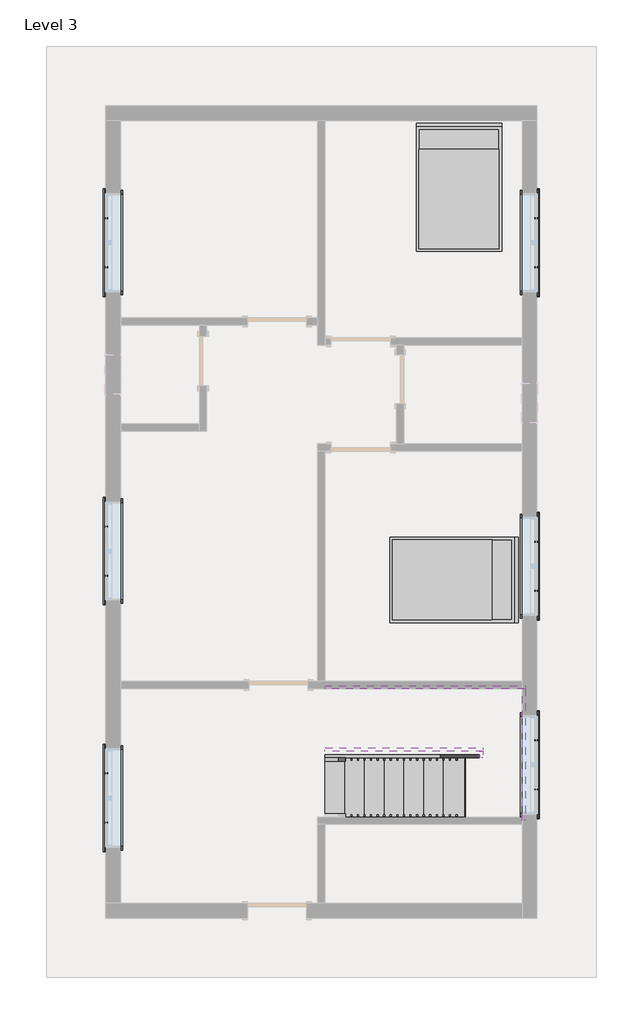
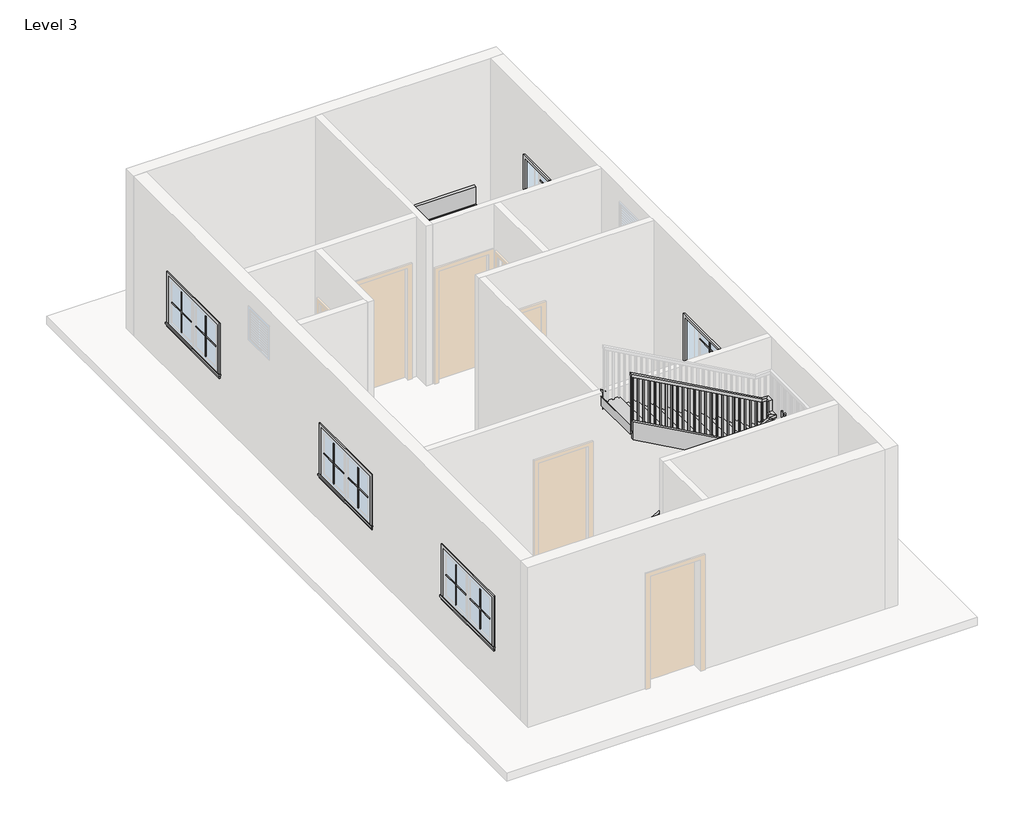
# One storey, part 3 of 3: 24 proxies, 6 members, 2 furniture elements, 1 railing, 1 stair flight.
"""IFC4 building model written with IfcOpenShell, lengths in millimetres."""

from ifc_helpers import new_model, si_unit, frame, origin, place, context, project, spatial, polyline, outline, extrude, faceted_brep, transform, mapped, element, save
from components import muntin_pattern_2x2_muntin_pattern_2x2_9352d081, muntin_pattern_2x2_muntin_pattern_2x2_5c2cbe28, trim_window_exterior_flat_with_sill_979bde60, trim_window_interior_flat_picture_frame_7883d11b, bed_17739_bed_17739_15c61121, stair_flight_460b4896

model = new_model("IFC4")

# Units and contexts
model_context = context("Model", 3, world=origin())
ifc_project = project(units=[si_unit("LENGTHUNIT", "METRE", prefix="MILLI")], contexts=[model_context])

# Site, building, storey
site = spatial("IfcSite", under=ifc_project)
building = spatial("IfcBuilding", under=site)
storey = spatial("IfcBuildingStorey", under=building, Name="Level 3", Elevation=6248.4)

# Proxies
placement = place(None, origin())
muntin_pattern_2x2_muntin_pattern_2x2_shape = muntin_pattern_2x2_muntin_pattern_2x2_9352d081(model_context)
element("IfcBuildingElementProxy", 1, Name="Muntin Pattern_2x2 : Muntin Pattern_2x2", ObjectType="Muntin Pattern_2x2 : Muntin Pattern_2x2", at=placement, inside=storey, context=model_context, shape_type="MappedRepresentation", body=[
    mapped(muntin_pattern_2x2_muntin_pattern_2x2_shape, transform((-4579.34688, 3675.02881, 7232.65), x_axis=(0.0, 1.0, 0.0), y_axis=(-1.0, 0.0, 0.0), z_axis=(0.0, 0.0, 1.0))),
])
element("IfcBuildingElementProxy", 2, Name="Muntin Pattern_2x2 : Muntin Pattern_2x2", ObjectType="Muntin Pattern_2x2 : Muntin Pattern_2x2", at=placement, inside=storey, context=model_context, shape_type="MappedRepresentation", body=[
    mapped(muntin_pattern_2x2_muntin_pattern_2x2_shape, transform((-4579.34688, -1087.47119, 7232.65), x_axis=(0.0, 1.0, 0.0), y_axis=(-1.0, 0.0, 0.0), z_axis=(0.0, 0.0, 1.0))),
])
element("IfcBuildingElementProxy", 3, Name="Muntin Pattern_2x2 : Muntin Pattern_2x2", ObjectType="Muntin Pattern_2x2 : Muntin Pattern_2x2", at=placement, inside=storey, context=model_context, shape_type="MappedRepresentation", body=[
    mapped(muntin_pattern_2x2_muntin_pattern_2x2_shape, transform((-4579.34688, -4900.64619, 7232.65), x_axis=(0.0, 1.0, 0.0), y_axis=(-1.0, 0.0, 0.0), z_axis=(0.0, 0.0, 1.0))),
])
element("IfcBuildingElementProxy", 4, Name="Muntin Pattern_2x2 : Muntin Pattern_2x2", ObjectType="Muntin Pattern_2x2 : Muntin Pattern_2x2", at=placement, inside=storey, context=model_context, shape_type="MappedRepresentation", body=[
    mapped(muntin_pattern_2x2_muntin_pattern_2x2_shape, transform((2069.10312, -3630.64619, 7232.65), x_axis=(0.0, -1.0, 0.0), y_axis=(1.0, 0.0, 0.0), z_axis=(0.0, 0.0, 1.0))),
])
element("IfcBuildingElementProxy", 5, Name="Muntin Pattern_2x2 : Muntin Pattern_2x2", ObjectType="Muntin Pattern_2x2 : Muntin Pattern_2x2", at=placement, inside=storey, context=model_context, shape_type="MappedRepresentation", body=[
    mapped(muntin_pattern_2x2_muntin_pattern_2x2_shape, transform((2069.10312, 4433.85381, 7232.65), x_axis=(0.0, -1.0, 0.0), y_axis=(1.0, 0.0, 0.0), z_axis=(0.0, 0.0, 1.0))),
])
element("IfcBuildingElementProxy", 6, Name="Muntin Pattern_2x2 : Muntin Pattern_2x2", ObjectType="Muntin Pattern_2x2 : Muntin Pattern_2x2", at=placement, inside=storey, context=model_context, shape_type="MappedRepresentation", body=[
    mapped(muntin_pattern_2x2_muntin_pattern_2x2_shape, transform((2069.10312, -563.59619, 7232.65), x_axis=(0.0, -1.0, 0.0), y_axis=(1.0, 0.0, 0.0), z_axis=(0.0, 0.0, 1.0))),
])
muntin_pattern_2x2_muntin_pattern_2x2_2_shape = muntin_pattern_2x2_muntin_pattern_2x2_5c2cbe28(model_context)
element("IfcBuildingElementProxy", 7, Name="Muntin Pattern_2x2 : Muntin Pattern_2x2", ObjectType="Muntin Pattern_2x2 : Muntin Pattern_2x2", at=placement, inside=storey, context=model_context, shape_type="MappedRepresentation", body=[
    mapped(muntin_pattern_2x2_muntin_pattern_2x2_2_shape, transform((-4579.34688, 4433.85381, 7232.65), x_axis=(0.0, -1.0, 0.0), y_axis=(1.0, 0.0, 0.0), z_axis=(0.0, 0.0, 1.0))),
])
element("IfcBuildingElementProxy", 8, Name="Muntin Pattern_2x2 : Muntin Pattern_2x2", ObjectType="Muntin Pattern_2x2 : Muntin Pattern_2x2", at=placement, inside=storey, context=model_context, shape_type="MappedRepresentation", body=[
    mapped(muntin_pattern_2x2_muntin_pattern_2x2_2_shape, transform((-4579.34688, -328.64619, 7232.65), x_axis=(0.0, -1.0, 0.0), y_axis=(1.0, 0.0, 0.0), z_axis=(0.0, 0.0, 1.0))),
])
element("IfcBuildingElementProxy", 9, Name="Muntin Pattern_2x2 : Muntin Pattern_2x2", ObjectType="Muntin Pattern_2x2 : Muntin Pattern_2x2", at=placement, inside=storey, context=model_context, shape_type="MappedRepresentation", body=[
    mapped(muntin_pattern_2x2_muntin_pattern_2x2_2_shape, transform((-4579.34688, -4141.82119, 7232.65), x_axis=(0.0, -1.0, 0.0), y_axis=(1.0, 0.0, 0.0), z_axis=(0.0, 0.0, 1.0))),
])
element("IfcBuildingElementProxy", 10, Name="Muntin Pattern_2x2 : Muntin Pattern_2x2", ObjectType="Muntin Pattern_2x2 : Muntin Pattern_2x2", at=placement, inside=storey, context=model_context, shape_type="MappedRepresentation", body=[
    mapped(muntin_pattern_2x2_muntin_pattern_2x2_2_shape, transform((2069.10312, -4389.47119, 7232.65), x_axis=(0.0, 1.0, 0.0), y_axis=(-1.0, 0.0, 0.0), z_axis=(0.0, 0.0, 1.0))),
])
element("IfcBuildingElementProxy", 11, Name="Muntin Pattern_2x2 : Muntin Pattern_2x2", ObjectType="Muntin Pattern_2x2 : Muntin Pattern_2x2", at=placement, inside=storey, context=model_context, shape_type="MappedRepresentation", body=[
    mapped(muntin_pattern_2x2_muntin_pattern_2x2_2_shape, transform((2069.10312, 3675.02881, 7232.65), x_axis=(0.0, 1.0, 0.0), y_axis=(-1.0, 0.0, 0.0), z_axis=(0.0, 0.0, 1.0))),
])
element("IfcBuildingElementProxy", 12, Name="Muntin Pattern_2x2 : Muntin Pattern_2x2", ObjectType="Muntin Pattern_2x2 : Muntin Pattern_2x2", at=placement, inside=storey, context=model_context, shape_type="MappedRepresentation", body=[
    mapped(muntin_pattern_2x2_muntin_pattern_2x2_2_shape, transform((2069.10312, -1322.42119, 7232.65), x_axis=(0.0, 1.0, 0.0), y_axis=(-1.0, 0.0, 0.0), z_axis=(0.0, 0.0, 1.0))),
])
trim_window_exterior_flat_with_sill_shape = trim_window_exterior_flat_with_sill_979bde60(model_context)
element("IfcBuildingElementProxy", 13, Name="Trim-Window-Exterior-Flat : with Sill", ObjectType="Trim-Window-Exterior-Flat : with Sill", at=placement, inside=storey, context=model_context, shape_type="MappedRepresentation", body=[
    mapped(trim_window_exterior_flat_with_sill_shape, transform((-4588.87188, 4054.44131, 8077.2), x_axis=(0.0, -1.0, 0.0), y_axis=(0.0, 0.0, 1.0), z_axis=(-1.0, 0.0, 0.0))),
])
element("IfcBuildingElementProxy", 14, Name="Trim-Window-Exterior-Flat : with Sill", ObjectType="Trim-Window-Exterior-Flat : with Sill", at=placement, inside=storey, context=model_context, shape_type="MappedRepresentation", body=[
    mapped(trim_window_exterior_flat_with_sill_shape, transform((-4588.87188, -708.05869, 8077.2), x_axis=(0.0, -1.0, 0.0), y_axis=(0.0, 0.0, 1.0), z_axis=(-1.0, 0.0, 0.0))),
])
element("IfcBuildingElementProxy", 15, Name="Trim-Window-Exterior-Flat : with Sill", ObjectType="Trim-Window-Exterior-Flat : with Sill", at=placement, inside=storey, context=model_context, shape_type="MappedRepresentation", body=[
    mapped(trim_window_exterior_flat_with_sill_shape, transform((-4588.87188, -4521.23369, 8077.2), x_axis=(0.0, -1.0, 0.0), y_axis=(0.0, 0.0, 1.0), z_axis=(-1.0, 0.0, 0.0))),
])
element("IfcBuildingElementProxy", 16, Name="Trim-Window-Exterior-Flat : with Sill", ObjectType="Trim-Window-Exterior-Flat : with Sill", at=placement, inside=storey, context=model_context, shape_type="MappedRepresentation", body=[
    mapped(trim_window_exterior_flat_with_sill_shape, transform((2078.62812, -4010.05869, 8077.2), x_axis=(0.0, 1.0, 0.0), y_axis=(0.0, 0.0, 1.0), z_axis=(1.0, 0.0, 0.0))),
])
element("IfcBuildingElementProxy", 17, Name="Trim-Window-Exterior-Flat : with Sill", ObjectType="Trim-Window-Exterior-Flat : with Sill", at=placement, inside=storey, context=model_context, shape_type="MappedRepresentation", body=[
    mapped(trim_window_exterior_flat_with_sill_shape, transform((2078.62812, 4054.44131, 8077.2), x_axis=(0.0, 1.0, 0.0), y_axis=(0.0, 0.0, 1.0), z_axis=(1.0, 0.0, 0.0))),
])
element("IfcBuildingElementProxy", 18, Name="Trim-Window-Exterior-Flat : with Sill", ObjectType="Trim-Window-Exterior-Flat : with Sill", at=placement, inside=storey, context=model_context, shape_type="MappedRepresentation", body=[
    mapped(trim_window_exterior_flat_with_sill_shape, transform((2078.62812, -943.00869, 8077.2), x_axis=(0.0, 1.0, 0.0), y_axis=(0.0, 0.0, 1.0), z_axis=(1.0, 0.0, 0.0))),
])
trim_window_interior_flat_picture_frame_shape = trim_window_interior_flat_picture_frame_7883d11b(model_context)
element("IfcBuildingElementProxy", 19, Name="Trim-Window-Interior-Flat : Picture Frame", ObjectType="Trim-Window-Interior-Flat : Picture Frame", at=placement, inside=storey, context=model_context, shape_type="MappedRepresentation", body=[
    mapped(trim_window_interior_flat_picture_frame_shape, transform((-4360.27188, 4054.44131, 8077.2), x_axis=(0.0, 1.0, 0.0), y_axis=(0.0, 0.0, 1.0), z_axis=(1.0, 0.0, 0.0))),
])
element("IfcBuildingElementProxy", 20, Name="Trim-Window-Interior-Flat : Picture Frame", ObjectType="Trim-Window-Interior-Flat : Picture Frame", at=placement, inside=storey, context=model_context, shape_type="MappedRepresentation", body=[
    mapped(trim_window_interior_flat_picture_frame_shape, transform((-4360.27188, -708.05869, 8077.2), x_axis=(0.0, 1.0, 0.0), y_axis=(0.0, 0.0, 1.0), z_axis=(1.0, 0.0, 0.0))),
])
element("IfcBuildingElementProxy", 21, Name="Trim-Window-Interior-Flat : Picture Frame", ObjectType="Trim-Window-Interior-Flat : Picture Frame", at=placement, inside=storey, context=model_context, shape_type="MappedRepresentation", body=[
    mapped(trim_window_interior_flat_picture_frame_shape, transform((-4360.27188, -4521.23369, 8077.2), x_axis=(0.0, 1.0, 0.0), y_axis=(0.0, 0.0, 1.0), z_axis=(1.0, 0.0, 0.0))),
])
element("IfcBuildingElementProxy", 22, Name="Trim-Window-Interior-Flat : Picture Frame", ObjectType="Trim-Window-Interior-Flat : Picture Frame", at=placement, inside=storey, context=model_context, shape_type="MappedRepresentation", body=[
    mapped(trim_window_interior_flat_picture_frame_shape, transform((1850.02812, -4010.05869, 8077.2), x_axis=(0.0, -1.0, 0.0), y_axis=(0.0, 0.0, 1.0), z_axis=(-1.0, 0.0, 0.0))),
])
element("IfcBuildingElementProxy", 23, Name="Trim-Window-Interior-Flat : Picture Frame", ObjectType="Trim-Window-Interior-Flat : Picture Frame", at=placement, inside=storey, context=model_context, shape_type="MappedRepresentation", body=[
    mapped(trim_window_interior_flat_picture_frame_shape, transform((1850.02812, 4054.44131, 8077.2), x_axis=(0.0, -1.0, 0.0), y_axis=(0.0, 0.0, 1.0), z_axis=(-1.0, 0.0, 0.0))),
])
element("IfcBuildingElementProxy", 24, Name="Trim-Window-Interior-Flat : Picture Frame", ObjectType="Trim-Window-Interior-Flat : Picture Frame", at=placement, inside=storey, context=model_context, shape_type="MappedRepresentation", body=[
    mapped(trim_window_interior_flat_picture_frame_shape, transform((1850.02812, -943.00869, 8077.2), x_axis=(0.0, -1.0, 0.0), y_axis=(0.0, 0.0, 1.0), z_axis=(-1.0, 0.0, 0.0))),
])

# Furniture
bed_17739_bed_17739_shape = bed_17739_bed_17739_15c61121(model_context)
element("IfcFurniture", 25, ObjectType="Bed_17739 : Bed_17739", at=placement, inside=storey, context=model_context, shape_type="MappedRepresentation", body=[
    mapped(bed_17739_bed_17739_shape, transform((872.12812, 4886.29131, 6248.4), x_axis=(1.0, 0.0, 0.0), y_axis=(0.0, 1.0, 0.0), z_axis=(0.0, 0.0, 1.0))),
])
element("IfcFurniture", 26, ObjectType="Bed_17739 : Bed_17739", at=placement, inside=storey, context=model_context, shape_type="MappedRepresentation", body=[
    mapped(bed_17739_bed_17739_shape, transform((770.52812, -1152.55869, 6248.4), x_axis=(0.0, -1.0, 0.0), y_axis=(1.0, 0.0, 0.0), z_axis=(0.0, 0.0, 1.0))),
])

# Members
element("IfcMember", 27, ObjectType="Stringer - 2\" Width", at=placement, inside=storey, context=model_context, shape_type="SweptSolid", body=[
    extrude(outline(polyline([(6455.9983948, -1197.97188), (6248.4, -1197.97188), (6248.4, -944.0273772), (7433.7641651, 1189.62812), (7782.4428392, 1189.62812), (6455.9983948, -1197.97188)])), frame((0.0, -3902.10869, 0.0), z_axis=(0.0, 1.0, 0.0), x_axis=(0.0, 0.0, 1.0)), (0.0, 0.0, 1.0), 50.8),
])
element("IfcMember", 28, ObjectType="Stringer - 2\" Width", at=placement, inside=storey, context=model_context, shape_type="SweptSolid", body=[
    extrude(outline(polyline([(1240.42812, -3902.10869), (1189.62812, -3902.10869), (1189.62812, -3800.50869), (1240.42812, -3800.50869), (1240.42812, -3902.10869)])), frame((0.0, 0.0, 7543.8), z_axis=(0.0, 0.0, 1.0), x_axis=(1.0, 0.0, 0.0)), (0.0, 0.0, 1.0), 304.8),
])
element("IfcMember", 29, ObjectType="Stringer - 2\" Width", at=placement, inside=storey, context=model_context, shape_type="SweptSolid", body=[
    extrude(outline(polyline([(7631.3197207, 1240.42812), (7979.9983948, 1240.42812), (9334.6650614, -1197.97188), (8985.9863873, -1197.97188), (7631.3197207, 1240.42812)])), frame((0.0, -3800.50869, 0.0), z_axis=(0.0, 1.0, 0.0), x_axis=(0.0, 0.0, 1.0)), (0.0, 0.0, 1.0), 50.8),
])
element("IfcMember", 30, ObjectType="Stringer - 2\" Width", at=placement, inside=storey, context=model_context, shape_type="SweptSolid", body=[
    extrude(outline(polyline([(6455.9983948, -1197.97188), (6248.4, -1197.97188), (6248.4, -944.0273772), (7800.653054, 1850.02812), (7848.6, 1850.02812), (7848.6, 1308.7110094), (6455.9983948, -1197.97188)])), frame((0.0, -4867.30869, 0.0), z_axis=(0.0, 1.0, 0.0), x_axis=(0.0, 0.0, 1.0)), (0.0, 0.0, 1.0), 50.8),
])
element("IfcMember", 31, ObjectType="Stringer - 2\" Width", at=placement, inside=storey, context=model_context, shape_type="SweptSolid", body=[
    extrude(outline(polyline([(1900.82812, -4867.30869), (1850.02812, -4867.30869), (1850.02812, -2835.30869), (1900.82812, -2835.30869), (1900.82812, -4867.30869)])), frame((0.0, 0.0, 7543.8), z_axis=(0.0, 0.0, 1.0), x_axis=(1.0, 0.0, 0.0)), (0.0, 0.0, 1.0), 304.8),
])
element("IfcMember", 32, ObjectType="Stringer - 2\" Width", at=placement, inside=storey, context=model_context, shape_type="SweptSolid", body=[
    extrude(outline(polyline([(7543.8, 1900.82812), (7613.1095059, 1900.82812), (9334.6650614, -1197.97188), (8985.9863873, -1197.97188), (7543.8, 1397.9636172), (7543.8, 1900.82812)])), frame((0.0, -2835.30869, 0.0), z_axis=(0.0, 1.0, 0.0), x_axis=(0.0, 0.0, 1.0)), (0.0, 0.0, 1.0), 50.8),
])

# Railing
element("IfcRailing", 33, ObjectType="Handrail - Rectangular", at=placement, inside=storey, context=model_context, shape_type="SolidModel", body=[
    faceted_brep([(-1197.97188, -3902.10869, 7332.1333333), (-1197.97188, -3902.10869, 7274.020221), (-1197.97188, -3952.90869, 7274.020221), (-1197.97188, -3952.90869, 7332.1333333), (1164.22812, -3902.10869, 8644.4666667), (1215.02812, -3902.10869, 8614.5757765), (1215.02812, -3952.90869, 8614.5757765), (1164.22812, -3952.90869, 8644.4666667), (1164.22812, -3902.10869, 8686.8), (1215.02812, -3902.10869, 8636.0), (1215.02812, -3952.90869, 8636.0), (1164.22812, -3952.90869, 8686.8), (1240.42812, -3902.10869, 8686.8), (1240.42812, -3902.10869, 8636.0), (1291.22812, -3952.90869, 8636.0), (1291.22812, -3952.90869, 8686.8), (1240.42812, -3825.90869, 8686.8), (1240.42812, -3775.10869, 8636.0), (1291.22812, -3775.10869, 8636.0), (1291.22812, -3825.90869, 8686.8), (1240.42812, -3825.90869, 8898.4666667), (1240.42812, -3775.10869, 8847.6666667), (1291.22812, -3775.10869, 8847.6666667), (1291.22812, -3825.90869, 8898.4666667), (1240.42812, -3749.70869, 8898.4666667), (1240.42812, -3749.70869, 8847.6666667), (1291.22812, -3698.90869, 8847.6666667), (1291.22812, -3698.90869, 8898.4666667), (1164.22812, -3749.70869, 8898.4666667), (1151.0645177, -3749.70869, 8847.6666667), (1151.0645177, -3698.90869, 8847.6666667), (1164.22812, -3698.90869, 8898.4666667), (-1197.97188, -3749.70869, 10210.8), (-1197.97188, -3698.90869, 10210.8), (-1197.97188, -3698.90869, 10152.6868876), (-1197.97188, -3749.70869, 10152.6868876)], [[[0, 1, 2, 3]], [[1, 0, 4, 5]], [[2, 1, 5, 6]], [[3, 2, 6, 7]], [[0, 3, 7, 4]], [[5, 4, 8, 9]], [[6, 5, 9, 10]], [[7, 6, 10, 11]], [[4, 7, 11, 8]], [[9, 8, 12, 13]], [[10, 9, 13, 14]], [[11, 10, 14, 15]], [[8, 11, 15, 12]], [[13, 12, 16, 17]], [[14, 13, 17, 18]], [[15, 14, 18, 19]], [[12, 15, 19, 16]], [[17, 16, 20, 21]], [[18, 17, 21, 22]], [[19, 18, 22, 23]], [[16, 19, 23, 20]], [[21, 20, 24, 25]], [[22, 21, 25, 26]], [[23, 22, 26, 27]], [[20, 23, 27, 24]], [[25, 24, 28, 29]], [[26, 25, 29, 30]], [[27, 26, 30, 31]], [[24, 27, 31, 28]], [[32, 33, 34, 35]], [[29, 28, 32, 35]], [[30, 29, 35, 34]], [[31, 30, 34, 33]], [[28, 31, 33, 32]]]),
    extrude(outline(polyline([(10143.8674432, -1182.09688), (9127.0666667, -1182.09688), (9127.0666667, -1163.04688), (10133.2841099, -1163.04688), (10143.8674432, -1182.09688)])), frame((0.0, -3733.83369, 0.0), z_axis=(0.0, 1.0, 0.0), x_axis=(0.0, 0.0, 1.0)), (0.0, 0.0, 1.0), 19.05),
    extrude(outline(polyline([(10087.4229988, -1080.49688), (9127.0666667, -1080.49688), (9127.0666667, -1061.44688), (10076.8396654, -1061.44688), (10087.4229988, -1080.49688)])), frame((0.0, -3733.83369, 0.0), z_axis=(0.0, 1.0, 0.0), x_axis=(0.0, 0.0, 1.0)), (0.0, 0.0, 1.0), 19.05),
    extrude(outline(polyline([(10030.9785543, -978.89688), (9127.0666667, -978.89688), (9127.0666667, -959.84688), (10020.395221, -959.84688), (10030.9785543, -978.89688)])), frame((0.0, -3733.83369, 0.0), z_axis=(0.0, 1.0, 0.0), x_axis=(0.0, 0.0, 1.0)), (0.0, 0.0, 1.0), 19.05),
    extrude(outline(polyline([(9974.5341099, -877.29688), (8957.7333333, -877.29688), (8957.7333333, -858.24688), (9963.9507765, -858.24688), (9974.5341099, -877.29688)])), frame((0.0, -3733.83369, 0.0), z_axis=(0.0, 1.0, 0.0), x_axis=(0.0, 0.0, 1.0)), (0.0, 0.0, 1.0), 19.05),
    extrude(outline(polyline([(9918.0896654, -775.69688), (8957.7333333, -775.69688), (8957.7333333, -756.64688), (9907.5063321, -756.64688), (9918.0896654, -775.69688)])), frame((0.0, -3733.83369, 0.0), z_axis=(0.0, 1.0, 0.0), x_axis=(0.0, 0.0, 1.0)), (0.0, 0.0, 1.0), 19.05),
    extrude(outline(polyline([(9861.645221, -674.09688), (8957.7333333, -674.09688), (8957.7333333, -655.04688), (9851.0618876, -655.04688), (9861.645221, -674.09688)])), frame((0.0, -3733.83369, 0.0), z_axis=(0.0, 1.0, 0.0), x_axis=(0.0, 0.0, 1.0)), (0.0, 0.0, 1.0), 19.05),
    extrude(outline(polyline([(9805.2007765, -572.49688), (8788.4, -572.49688), (8788.4, -553.44688), (9794.6174432, -553.44688), (9805.2007765, -572.49688)])), frame((0.0, -3733.83369, 0.0), z_axis=(0.0, 1.0, 0.0), x_axis=(0.0, 0.0, 1.0)), (0.0, 0.0, 1.0), 19.05),
    extrude(outline(polyline([(9748.7563321, -470.89688), (8788.4, -470.89688), (8788.4, -451.84688), (9738.1729988, -451.84688), (9748.7563321, -470.89688)])), frame((0.0, -3733.83369, 0.0), z_axis=(0.0, 1.0, 0.0), x_axis=(0.0, 0.0, 1.0)), (0.0, 0.0, 1.0), 19.05),
    extrude(outline(polyline([(9692.3118876, -369.29688), (8788.4, -369.29688), (8788.4, -350.24688), (9681.7285543, -350.24688), (9692.3118876, -369.29688)])), frame((0.0, -3733.83369, 0.0), z_axis=(0.0, 1.0, 0.0), x_axis=(0.0, 0.0, 1.0)), (0.0, 0.0, 1.0), 19.05),
    extrude(outline(polyline([(9635.8674432, -267.69688), (8619.0666667, -267.69688), (8619.0666667, -248.64688), (9625.2841099, -248.64688), (9635.8674432, -267.69688)])), frame((0.0, -3733.83369, 0.0), z_axis=(0.0, 1.0, 0.0), x_axis=(0.0, 0.0, 1.0)), (0.0, 0.0, 1.0), 19.05),
    extrude(outline(polyline([(9579.4229988, -166.09688), (8619.0666667, -166.09688), (8619.0666667, -147.04688), (9568.8396654, -147.04688), (9579.4229988, -166.09688)])), frame((0.0, -3733.83369, 0.0), z_axis=(0.0, 1.0, 0.0), x_axis=(0.0, 0.0, 1.0)), (0.0, 0.0, 1.0), 19.05),
    extrude(outline(polyline([(9522.9785543, -64.49688), (8619.0666667, -64.49688), (8619.0666667, -45.44688), (9512.395221, -45.44688), (9522.9785543, -64.49688)])), frame((0.0, -3733.83369, 0.0), z_axis=(0.0, 1.0, 0.0), x_axis=(0.0, 0.0, 1.0)), (0.0, 0.0, 1.0), 19.05),
    extrude(outline(polyline([(9466.5341099, 37.10312), (8449.7333333, 37.10312), (8449.7333333, 56.15312), (9455.9507765, 56.15312), (9466.5341099, 37.10312)])), frame((0.0, -3733.83369, 0.0), z_axis=(0.0, 1.0, 0.0), x_axis=(0.0, 0.0, 1.0)), (0.0, 0.0, 1.0), 19.05),
    extrude(outline(polyline([(9410.0896654, 138.70312), (8449.7333333, 138.70312), (8449.7333333, 157.75312), (9399.5063321, 157.75312), (9410.0896654, 138.70312)])), frame((0.0, -3733.83369, 0.0), z_axis=(0.0, 1.0, 0.0), x_axis=(0.0, 0.0, 1.0)), (0.0, 0.0, 1.0), 19.05),
    extrude(outline(polyline([(9353.645221, 240.30312), (8449.7333333, 240.30312), (8449.7333333, 259.35312), (9343.0618876, 259.35312), (9353.645221, 240.30312)])), frame((0.0, -3733.83369, 0.0), z_axis=(0.0, 1.0, 0.0), x_axis=(0.0, 0.0, 1.0)), (0.0, 0.0, 1.0), 19.05),
    extrude(outline(polyline([(9297.2007765, 341.90312), (8280.4, 341.90312), (8280.4, 360.95312), (9286.6174432, 360.95312), (9297.2007765, 341.90312)])), frame((0.0, -3733.83369, 0.0), z_axis=(0.0, 1.0, 0.0), x_axis=(0.0, 0.0, 1.0)), (0.0, 0.0, 1.0), 19.05),
    extrude(outline(polyline([(9240.7563321, 443.50312), (8280.4, 443.50312), (8280.4, 462.55312), (9230.1729988, 462.55312), (9240.7563321, 443.50312)])), frame((0.0, -3733.83369, 0.0), z_axis=(0.0, 1.0, 0.0), x_axis=(0.0, 0.0, 1.0)), (0.0, 0.0, 1.0), 19.05),
    extrude(outline(polyline([(9184.3118876, 545.10312), (8280.4, 545.10312), (8280.4, 564.15312), (9173.7285543, 564.15312), (9184.3118876, 545.10312)])), frame((0.0, -3733.83369, 0.0), z_axis=(0.0, 1.0, 0.0), x_axis=(0.0, 0.0, 1.0)), (0.0, 0.0, 1.0), 19.05),
    extrude(outline(polyline([(9127.8674432, 646.70312), (8111.0666667, 646.70312), (8111.0666667, 665.75312), (9117.2841099, 665.75312), (9127.8674432, 646.70312)])), frame((0.0, -3733.83369, 0.0), z_axis=(0.0, 1.0, 0.0), x_axis=(0.0, 0.0, 1.0)), (0.0, 0.0, 1.0), 19.05),
    extrude(outline(polyline([(9071.4229988, 748.30312), (8111.0666667, 748.30312), (8111.0666667, 767.35312), (9060.8396654, 767.35312), (9071.4229988, 748.30312)])), frame((0.0, -3733.83369, 0.0), z_axis=(0.0, 1.0, 0.0), x_axis=(0.0, 0.0, 1.0)), (0.0, 0.0, 1.0), 19.05),
    extrude(outline(polyline([(9014.9785543, 849.90312), (8111.0666667, 849.90312), (8111.0666667, 868.95312), (9004.395221, 868.95312), (9014.9785543, 849.90312)])), frame((0.0, -3733.83369, 0.0), z_axis=(0.0, 1.0, 0.0), x_axis=(0.0, 0.0, 1.0)), (0.0, 0.0, 1.0), 19.05),
    extrude(outline(polyline([(8958.5341099, 951.50312), (7941.7333333, 951.50312), (7941.7333333, 970.55312), (8947.9507765, 970.55312), (8958.5341099, 951.50312)])), frame((0.0, -3733.83369, 0.0), z_axis=(0.0, 1.0, 0.0), x_axis=(0.0, 0.0, 1.0)), (0.0, 0.0, 1.0), 19.05),
    extrude(outline(polyline([(8902.0896654, 1053.10312), (7941.7333333, 1053.10312), (7941.7333333, 1072.15312), (8891.5063321, 1072.15312), (8902.0896654, 1053.10312)])), frame((0.0, -3733.83369, 0.0), z_axis=(0.0, 1.0, 0.0), x_axis=(0.0, 0.0, 1.0)), (0.0, 0.0, 1.0), 19.05),
    extrude(outline(polyline([(8845.645221, 1154.70312), (7941.7333333, 1154.70312), (7941.7333333, 1173.75312), (8835.0618876, 1173.75312), (8845.645221, 1154.70312)])), frame((0.0, -3733.83369, 0.0), z_axis=(0.0, 1.0, 0.0), x_axis=(0.0, 0.0, 1.0)), (0.0, 0.0, 1.0), 19.05),
    extrude(outline(polyline([(1256.30312, -3835.43369), (1256.30312, -3816.38369), (1275.35312, -3816.38369), (1275.35312, -3835.43369), (1256.30312, -3835.43369)])), frame((0.0, 0.0, 7772.4), z_axis=(0.0, 0.0, 1.0), x_axis=(1.0, 0.0, 0.0)), (0.0, 0.0, 1.0), 863.6),
    extrude(outline(polyline([(1230.90312, -3917.98369), (1249.95312, -3917.98369), (1249.95312, -3937.03369), (1230.90312, -3937.03369), (1230.90312, -3917.98369)])), frame((0.0, 0.0, 7772.4), z_axis=(0.0, 0.0, 1.0), x_axis=(1.0, 0.0, 0.0)), (0.0, 0.0, 1.0), 863.6),
    extrude(outline(polyline([(8566.9507765, 1129.30312), (7603.0666667, 1129.30312), (7603.0666667, 1148.35312), (8577.5341099, 1148.35312), (8566.9507765, 1129.30312)])), frame((0.0, -3937.03369, 0.0), z_axis=(0.0, 1.0, 0.0), x_axis=(0.0, 0.0, 1.0)), (0.0, 0.0, 1.0), 19.05),
    extrude(outline(polyline([(8510.5063321, 1027.70312), (7603.0666667, 1027.70312), (7603.0666667, 1046.75312), (8521.0896654, 1046.75312), (8510.5063321, 1027.70312)])), frame((0.0, -3937.03369, 0.0), z_axis=(0.0, 1.0, 0.0), x_axis=(0.0, 0.0, 1.0)), (0.0, 0.0, 1.0), 19.05),
    extrude(outline(polyline([(8454.0618876, 926.10312), (7603.0666667, 926.10312), (7603.0666667, 945.15312), (8464.645221, 945.15312), (8454.0618876, 926.10312)])), frame((0.0, -3937.03369, 0.0), z_axis=(0.0, 1.0, 0.0), x_axis=(0.0, 0.0, 1.0)), (0.0, 0.0, 1.0), 19.05),
    extrude(outline(polyline([(8397.6174432, 824.50312), (7433.7333333, 824.50312), (7433.7333333, 843.55312), (8408.2007765, 843.55312), (8397.6174432, 824.50312)])), frame((0.0, -3937.03369, 0.0), z_axis=(0.0, 1.0, 0.0), x_axis=(0.0, 0.0, 1.0)), (0.0, 0.0, 1.0), 19.05),
    extrude(outline(polyline([(8341.1729988, 722.90312), (7433.7333333, 722.90312), (7433.7333333, 741.95312), (8351.7563321, 741.95312), (8341.1729988, 722.90312)])), frame((0.0, -3937.03369, 0.0), z_axis=(0.0, 1.0, 0.0), x_axis=(0.0, 0.0, 1.0)), (0.0, 0.0, 1.0), 19.05),
    extrude(outline(polyline([(8284.7285543, 621.30312), (7433.7333333, 621.30312), (7433.7333333, 640.35312), (8295.3118876, 640.35312), (8284.7285543, 621.30312)])), frame((0.0, -3937.03369, 0.0), z_axis=(0.0, 1.0, 0.0), x_axis=(0.0, 0.0, 1.0)), (0.0, 0.0, 1.0), 19.05),
    extrude(outline(polyline([(8228.2841099, 519.70312), (7264.4, 519.70312), (7264.4, 538.75312), (8238.8674432, 538.75312), (8228.2841099, 519.70312)])), frame((0.0, -3937.03369, 0.0), z_axis=(0.0, 1.0, 0.0), x_axis=(0.0, 0.0, 1.0)), (0.0, 0.0, 1.0), 19.05),
    extrude(outline(polyline([(8171.8396654, 418.10312), (7264.4, 418.10312), (7264.4, 437.15312), (8182.4229988, 437.15312), (8171.8396654, 418.10312)])), frame((0.0, -3937.03369, 0.0), z_axis=(0.0, 1.0, 0.0), x_axis=(0.0, 0.0, 1.0)), (0.0, 0.0, 1.0), 19.05),
    extrude(outline(polyline([(8115.395221, 316.50312), (7264.4, 316.50312), (7264.4, 335.55312), (8125.9785543, 335.55312), (8115.395221, 316.50312)])), frame((0.0, -3937.03369, 0.0), z_axis=(0.0, 1.0, 0.0), x_axis=(0.0, 0.0, 1.0)), (0.0, 0.0, 1.0), 19.05),
    extrude(outline(polyline([(8058.9507765, 214.90312), (7095.0666667, 214.90312), (7095.0666667, 233.95312), (8069.5341099, 233.95312), (8058.9507765, 214.90312)])), frame((0.0, -3937.03369, 0.0), z_axis=(0.0, 1.0, 0.0), x_axis=(0.0, 0.0, 1.0)), (0.0, 0.0, 1.0), 19.05),
    extrude(outline(polyline([(8002.5063321, 113.30312), (7095.0666667, 113.30312), (7095.0666667, 132.35312), (8013.0896654, 132.35312), (8002.5063321, 113.30312)])), frame((0.0, -3937.03369, 0.0), z_axis=(0.0, 1.0, 0.0), x_axis=(0.0, 0.0, 1.0)), (0.0, 0.0, 1.0), 19.05),
    extrude(outline(polyline([(7946.0618876, 11.70312), (7095.0666667, 11.70312), (7095.0666667, 30.75312), (7956.645221, 30.75312), (7946.0618876, 11.70312)])), frame((0.0, -3937.03369, 0.0), z_axis=(0.0, 1.0, 0.0), x_axis=(0.0, 0.0, 1.0)), (0.0, 0.0, 1.0), 19.05),
    extrude(outline(polyline([(7889.6174432, -89.89688), (6925.7333333, -89.89688), (6925.7333333, -70.84688), (7900.2007765, -70.84688), (7889.6174432, -89.89688)])), frame((0.0, -3937.03369, 0.0), z_axis=(0.0, 1.0, 0.0), x_axis=(0.0, 0.0, 1.0)), (0.0, 0.0, 1.0), 19.05),
    extrude(outline(polyline([(7833.1729988, -191.49688), (6925.7333333, -191.49688), (6925.7333333, -172.44688), (7843.7563321, -172.44688), (7833.1729988, -191.49688)])), frame((0.0, -3937.03369, 0.0), z_axis=(0.0, 1.0, 0.0), x_axis=(0.0, 0.0, 1.0)), (0.0, 0.0, 1.0), 19.05),
    extrude(outline(polyline([(7776.7285543, -293.09688), (6925.7333333, -293.09688), (6925.7333333, -274.04688), (7787.3118876, -274.04688), (7776.7285543, -293.09688)])), frame((0.0, -3937.03369, 0.0), z_axis=(0.0, 1.0, 0.0), x_axis=(0.0, 0.0, 1.0)), (0.0, 0.0, 1.0), 19.05),
    extrude(outline(polyline([(7720.2841099, -394.69688), (6756.4, -394.69688), (6756.4, -375.64688), (7730.8674432, -375.64688), (7720.2841099, -394.69688)])), frame((0.0, -3937.03369, 0.0), z_axis=(0.0, 1.0, 0.0), x_axis=(0.0, 0.0, 1.0)), (0.0, 0.0, 1.0), 19.05),
    extrude(outline(polyline([(7663.8396654, -496.29688), (6756.4, -496.29688), (6756.4, -477.24688), (7674.4229988, -477.24688), (7663.8396654, -496.29688)])), frame((0.0, -3937.03369, 0.0), z_axis=(0.0, 1.0, 0.0), x_axis=(0.0, 0.0, 1.0)), (0.0, 0.0, 1.0), 19.05),
    extrude(outline(polyline([(7607.395221, -597.89688), (6756.4, -597.89688), (6756.4, -578.84688), (7617.9785543, -578.84688), (7607.395221, -597.89688)])), frame((0.0, -3937.03369, 0.0), z_axis=(0.0, 1.0, 0.0), x_axis=(0.0, 0.0, 1.0)), (0.0, 0.0, 1.0), 19.05),
    extrude(outline(polyline([(7550.9507765, -699.49688), (6587.0666667, -699.49688), (6587.0666667, -680.44688), (7561.5341099, -680.44688), (7550.9507765, -699.49688)])), frame((0.0, -3937.03369, 0.0), z_axis=(0.0, 1.0, 0.0), x_axis=(0.0, 0.0, 1.0)), (0.0, 0.0, 1.0), 19.05),
    extrude(outline(polyline([(7494.5063321, -801.09688), (6587.0666667, -801.09688), (6587.0666667, -782.04688), (7505.0896654, -782.04688), (7494.5063321, -801.09688)])), frame((0.0, -3937.03369, 0.0), z_axis=(0.0, 1.0, 0.0), x_axis=(0.0, 0.0, 1.0)), (0.0, 0.0, 1.0), 19.05),
    extrude(outline(polyline([(7438.0618876, -902.69688), (6587.0666667, -902.69688), (6587.0666667, -883.64688), (7448.645221, -883.64688), (7438.0618876, -902.69688)])), frame((0.0, -3937.03369, 0.0), z_axis=(0.0, 1.0, 0.0), x_axis=(0.0, 0.0, 1.0)), (0.0, 0.0, 1.0), 19.05),
    extrude(outline(polyline([(7381.6174432, -1004.29688), (6417.7333333, -1004.29688), (6417.7333333, -985.24688), (7392.2007765, -985.24688), (7381.6174432, -1004.29688)])), frame((0.0, -3937.03369, 0.0), z_axis=(0.0, 1.0, 0.0), x_axis=(0.0, 0.0, 1.0)), (0.0, 0.0, 1.0), 19.05),
    extrude(outline(polyline([(7325.1729988, -1105.89688), (6417.7333333, -1105.89688), (6417.7333333, -1086.84688), (7335.7563321, -1086.84688), (7325.1729988, -1105.89688)])), frame((0.0, -3937.03369, 0.0), z_axis=(0.0, 1.0, 0.0), x_axis=(0.0, 0.0, 1.0)), (0.0, 0.0, 1.0), 19.05),
    extrude(outline(polyline([(1256.30312, -3733.83369), (1256.30312, -3714.78369), (1275.35312, -3714.78369), (1275.35312, -3733.83369), (1256.30312, -3733.83369)])), frame((0.0, 0.0, 7772.4), z_axis=(0.0, 0.0, 1.0), x_axis=(1.0, 0.0, 0.0)), (0.0, 0.0, 1.0), 1075.2666667),
    extrude(outline(polyline([(1256.30312, -3917.98369), (1275.35312, -3917.98369), (1275.35312, -3937.03369), (1256.30312, -3937.03369), (1256.30312, -3917.98369)])), frame((0.0, 0.0, 7772.4), z_axis=(0.0, 0.0, 1.0), x_axis=(1.0, 0.0, 0.0)), (0.0, 0.0, 1.0), 863.6),
    extrude(outline(polyline([(10152.6868876, -1197.97188), (9127.0666667, -1197.97188), (9127.0666667, -1178.92188), (10142.1035543, -1178.92188), (10152.6868876, -1197.97188)])), frame((0.0, -3733.83369, 0.0), z_axis=(0.0, 1.0, 0.0), x_axis=(0.0, 0.0, 1.0)), (0.0, 0.0, 1.0), 19.05),
    extrude(outline(polyline([(7274.020221, -1197.97188), (6417.7333333, -1197.97188), (6417.7333333, -1178.92188), (7284.6035543, -1178.92188), (7274.020221, -1197.97188)])), frame((0.0, -3937.03369, 0.0), z_axis=(0.0, 1.0, 0.0), x_axis=(0.0, 0.0, 1.0)), (0.0, 0.0, 1.0), 19.05),
])

# Stair flight
stair_flight_shape = stair_flight_460b4896(model_context)
element("IfcStairFlight", 34, ObjectType="2\" Tread 1\" Nosing 1/4\" Riser", at=placement, inside=storey, context=model_context, shape_type="MappedRepresentation", body=[
    mapped(stair_flight_shape, transform((0.0, 0.0, 0.0), x_axis=(1.0, 0.0, 0.0), y_axis=(0.0, 1.0, 0.0), z_axis=(0.0, 0.0, 1.0))),
])

save(model, "model.ifc")

# Revit data of these elements
# Type "Muntin Pattern_2x2 : Muntin Pattern_2x2"
#   Width [instance default] = 4' - 0"
#   Thickness = 0' - 0 1/2"
#   Height [instance default] = 4' - 0"
#   Distance = 0' - 0 3/4"
#   Interior Material [instance default] = none
#   Exterior Material [instance default] = none
#   Default Elevation = 0
# Type "Trim-Window-Exterior-Flat : with Sill"
#   Trim Width = 0' - 2 1/4"
#   Trim Thickness_Picture Frame = 0' - 1 1/4"
#   Trim Thickness_with Sill = 0' - 0 3/4"
#   Sill Thickness = 0' - 1 1/4"
#   Opening Width [instance default] = 2' - 0"
#   Opening Height [instance default] = 3' - 0"
#   Default Elevation = 4' - 0"
#   Sill = yes
#   Picture Frame = no
#   Trim Material [instance default] = none
# Type "Trim-Window-Interior-Flat : Picture Frame"
#   Trim Thickness_Picture Frame = 0' - 1 1/4"
#   Trim Width = 0' - 2 1/4"
#   Trim Thickness_with Sill = 0' - 0 3/4"
#   Sill Thickness = 0' - 1 1/4"
#   Opening Width [instance default] = 2' - 0"
#   Opening Height [instance default] = 3' - 0"
#   Default Elevation = 4' - 0"
#   Sill = no
#   Picture Frame = yes
#   Trim Material [instance default] = none
# Type "Bed_17739 : Bed_17739"
#   Default Elevation = 0
# Type "Handrail - Rectangular"
#   Assembly Code = "C2010400"
#   built-in parameter 1008612 = 0.0416667 (stored number, unit not read)
#   built-in parameter 1008611 = 0.0416667 (stored number, unit not read)
#   built-in parameter 1008609 = 0.333333 (stored number, unit not read)
#   built-in parameter 1008604 = 0.166667 (stored number, unit not read)
#   built-in parameter 1008603 = 0.166667 (stored number, unit not read)
#   Railing Height = 3' - 0"
#   built-in parameter 1008630 = 2
#   built-in parameter 1008610 = 2
#   built-in parameter 1008618 = Baluster - Square : 3/4"
# Elements 1, 2, 3, 4, 5, 6, 7, 8, 9, 10, 11, 12 (IfcBuildingElementProxy, "Muntin Pattern_2x2 : Muntin Pattern_2x2")
#   Width = 2' - 0 5/8"
#   Height = 2' - 6 1/2"
#   Interior Material = Wood - Stained
#   Exterior Material = Clad - White
#   Phase Created = New Construction
#   Materials on its faces: "Clad - White", "Wood - Stained"
# Elements 13, 14, 15, 16, 17, 18 (IfcBuildingElementProxy, "Trim-Window-Exterior-Flat : with Sill")
#   Opening Width = 5' - 0"
#   Opening Height = 3' - 0"
#   Trim Material = Clad - White
#   Phase Created = New Construction
#   Materials on its faces: "Clad - White"
# Elements 19, 20, 21, 22, 23, 24 (IfcBuildingElementProxy, "Trim-Window-Interior-Flat : Picture Frame")
#   Opening Width = 5' - 0"
#   Opening Height = 3' - 0"
#   Trim Material = Wood - Stained
#   Phase Created = New Construction
#   Materials on its faces: "Wood - Stained"
# Elements 25, 26 (IfcFurniture, "Bed_17739 : Bed_17739")
#   Phase Created = New Construction
#   Materials on its faces: "legs", "sheets", "bed frame", "Blanket"
# Elements 27, 28, 29, 30, 31, 32 (IfcMember, "Stringer - 2\" Width")
#   Phase Created = New Construction
# Element 33 (IfcRailing, "Handrail - Rectangular")
#   Phase Created = New Construction
# Element 34 (IfcStairFlight, "2\" Tread 1\" Nosing 1/4\" Riser")
#   Phase Created = New Construction
# Materials
#   "Clad - White": class "Wood", colour RGB 242 242 238, transparency 0, Cost = 0
#   "Wood - Stained": class "Wood", colour RGB 224 178 126, transparency 0, Cost = 0
#   "legs": colour RGB 90 73 37, transparency 0, Cost = 0
#   "sheets": colour RGB 200 195 176, transparency 0, Cost = 0
#   "bed frame": colour RGB 90 73 37, transparency 0, Cost = 0
#   "Blanket": class "System", colour RGB 59 0 1, transparency 0, Cost = 0
